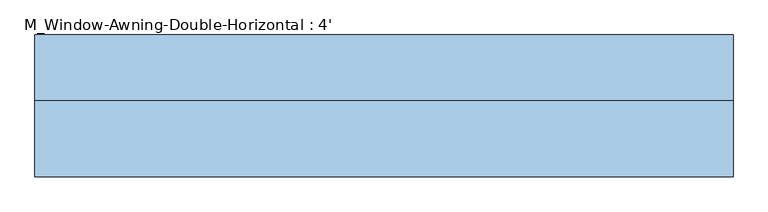
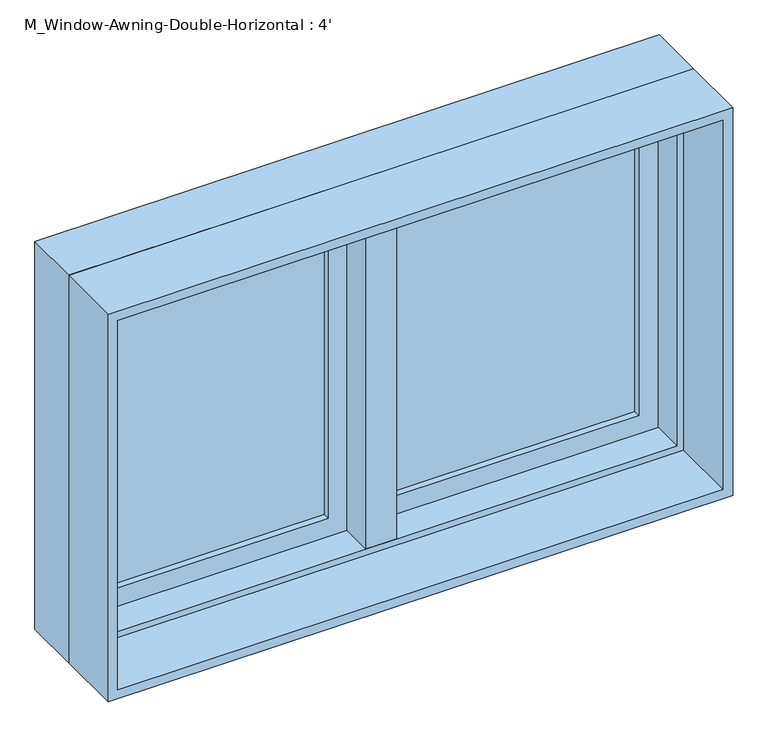
"""IFC4 building model written with IfcOpenShell, lengths in millimetres: window geometry, M_Window-Awning-Double-Horizontal : 4'."""

from ifc_helpers import new_model, si_unit, frame, origin, place, context, project, spatial, polyline, outline, extrude, faceted_brep, source, transform, mapped, element, save


def m_window_awning_double_horizontal_4_8afcb0b2(model_context):
    return source(origin(), model_context, "Body", "SolidModel", [
        faceted_brep([(577.85, 82.55, 1668.25), (577.85, 19.05, 1668.25), (-577.85, 19.05, 1668.25), (-577.85, 82.55, 1668.25), (596.9, 133.35, 1687.3), (596.9, 82.55, 1687.3), (-596.9, 82.55, 1687.3), (-596.9, 133.35, 1687.3), (609.6, 19.05, 1700.0), (609.6, 133.35, 1700.0), (-609.6, 133.35, 1700.0), (-609.6, 19.05, 1700.0), (-577.85, 19.05, 931.75), (-577.85, 82.55, 931.75), (-596.9, 82.55, 912.7), (-596.9, 133.35, 912.7), (-609.6, 133.35, 900.0), (-609.6, 19.05, 900.0), (577.85, 19.05, 931.75), (577.85, 82.55, 931.75), (596.9, 82.55, 912.7), (596.9, 133.35, 912.7), (609.6, 133.35, 900.0), (609.6, 19.05, 900.0)], [[[0, 1, 2, 3]], [[4, 5, 6, 7]], [[8, 9, 10, 11]], [[3, 2, 12, 13]], [[7, 6, 14, 15]], [[11, 10, 16, 17]], [[13, 12, 18, 19]], [[15, 14, 20, 21]], [[17, 16, 22, 23]], [[11, 17, 23, 8], [1, 18, 12, 2]], [[19, 18, 1, 0]], [[5, 20, 14, 6], [3, 13, 19, 0]], [[21, 20, 5, 4]], [[23, 22, 9, 8]], [[9, 22, 16, 10], [7, 15, 21, 4]]]),
        extrude(outline(polyline([(1700.0, -609.6), (900.0, -609.6), (900.0, 609.6), (1700.0, 609.6), (1700.0, -609.6)]), holes=[polyline([(1680.95, 590.55), (919.05, 590.55), (919.05, -590.55), (1680.95, -590.55), (1680.95, 590.55)])]), frame((0.0, -114.3, 0.0), z_axis=(0.0, 1.0, 0.0), x_axis=(0.0, 0.0, 1.0)), (0.0, 0.0, 1.0), 133.35),
        extrude(outline(polyline([(912.7, 596.9), (1687.3, 596.9), (1687.3, 9.525), (912.7, 9.525), (912.7, 596.9)]), holes=[polyline([(969.85, 66.675), (1630.15, 66.675), (1630.15, 539.75), (969.85, 539.75), (969.85, 66.675)])]), frame((0.0, 82.55, 0.0), z_axis=(0.0, 1.0, 0.0), x_axis=(0.0, 0.0, 1.0)), (0.0, 0.0, 1.0), 44.45),
        extrude(outline(polyline([(1687.3, -596.9), (912.7, -596.9), (912.7, -9.525), (1687.3, -9.525), (1687.3, -596.9)]), holes=[polyline([(1630.15, -66.675), (969.85, -66.675), (969.85, -539.75), (1630.15, -539.75), (1630.15, -66.675)])]), frame((0.0, 82.55, 0.0), z_axis=(0.0, 1.0, 0.0), x_axis=(0.0, 0.0, 1.0)), (0.0, 0.0, 1.0), 44.45),
        extrude(outline(polyline([(539.75, 114.3), (539.75, 107.95), (66.675, 107.95), (66.675, 114.3), (539.75, 114.3)])), frame((0.0, 0.0, 969.85), z_axis=(0.0, 0.0, 1.0), x_axis=(1.0, 0.0, 0.0)), (0.0, 0.0, 1.0), 660.3),
        extrude(outline(polyline([(66.675, 95.25), (66.675, 101.6), (539.75, 101.6), (539.75, 95.25), (66.675, 95.25)])), frame((0.0, 0.0, 969.85), z_axis=(0.0, 0.0, 1.0), x_axis=(1.0, 0.0, 0.0)), (0.0, 0.0, 1.0), 660.3),
        extrude(outline(polyline([(-66.675, 114.3), (-66.675, 107.95), (-539.75, 107.95), (-539.75, 114.3), (-66.675, 114.3)])), frame((0.0, 0.0, 969.85), z_axis=(0.0, 0.0, 1.0), x_axis=(1.0, 0.0, 0.0)), (0.0, 0.0, 1.0), 660.3),
        extrude(outline(polyline([(-539.75, 95.25), (-539.75, 101.6), (-66.675, 101.6), (-66.675, 95.25), (-539.75, 95.25)])), frame((0.0, 0.0, 969.85), z_axis=(0.0, 0.0, 1.0), x_axis=(1.0, 0.0, 0.0)), (0.0, 0.0, 1.0), 660.3),
        faceted_brep([(9.525, 133.35, 1687.3), (-9.525, 133.35, 1687.3), (-9.525, 82.55, 1687.3), (9.525, 82.55, 1687.3), (9.525, 133.35, 912.7), (9.525, 82.55, 912.7), (-9.525, 82.55, 912.7), (-9.525, 133.35, 912.7), (-9.525, 82.55, 931.75), (-9.525, 82.55, 1668.25), (-30.1625, 82.55, 931.75), (-30.1625, 82.55, 1668.25), (-30.1625, 19.05, 931.75), (-30.1625, 19.05, 1668.25), (30.1625, 19.05, 931.75), (30.1625, 19.05, 1668.25), (30.1625, 82.55, 931.75), (30.1625, 82.55, 1668.25), (9.525, 82.55, 931.75), (9.525, 82.55, 1668.25)], [[[0, 1, 2, 3]], [[4, 5, 6, 7]], [[1, 0, 4, 7]], [[2, 1, 7, 6, 8, 9]], [[9, 8, 10, 11]], [[11, 10, 12, 13]], [[13, 12, 14, 15]], [[15, 14, 16, 17]], [[17, 16, 18, 19]], [[0, 3, 19, 18, 5, 4]], [[18, 8, 6, 5]], [[9, 19, 3, 2]], [[8, 18, 16, 14, 12, 10]], [[19, 9, 11, 13, 15, 17]]]),
    ])


if __name__ == "__main__":
    model = new_model("IFC4")
    model_context = context("Model", 3, world=origin())
    ifc_project = project(units=[si_unit("LENGTHUNIT", "METRE", prefix="MILLI")], contexts=[model_context])
    site = spatial("IfcSite", under=ifc_project)
    building = spatial("IfcBuilding", under=site)
    placement = place(None, origin())
    m_window_awning_double_horizontal_4_shape = m_window_awning_double_horizontal_4_8afcb0b2(model_context)
    element("IfcWindow", 1, ObjectType="M_Window-Awning-Double-Horizontal : 4'", at=placement, inside=building, context=model_context, shape_type="MappedRepresentation", body=[
        mapped(m_window_awning_double_horizontal_4_shape, transform((0.0, 0.0, 0.0), x_axis=(1.0, 0.0, 0.0), y_axis=(0.0, 1.0, 0.0), z_axis=(0.0, 0.0, 1.0))),
    ])
    save(model, "model.ifc")

# Revit data of these elements
# Type "M_Window-Awning-Double-Horizontal : 4'"
#   Type Mark = "28"
#   Fire Rating = "0.5h"
#   Assembly Code = "B2020100"
#   Analytic Construction = "Double glazing - domestic"
#   Window Inset [instance default] = 0' - 0"
#   Wall Thickness [instance default] = 0' - 5.90551"
#   Interior Wall Closure [instance default] = 0' - 2.15551"
#   Half Width = 2' - 0"
#   Visual Light Transmittance = 0.81
#   Thermal Resistance (R) = 0.319569 (m²·K)/W
#   Solar Heat Gain Coefficient = 0.76
#   Rough Width = 4' - 0.59055"
#   Rough Height = 2' - 8.08661"
#   Height = 2' - 7.49606"
#   Heat Transfer Coefficient (U) = 3.12929 W/(m²·K)
#   Frame Extension [instance default] = 0' - 0 1/4"
#   Exterior Wall Closure [instance default] = 0' - 1 1/4"
#   Extension Jamb [instance default] = 0' - 2.15551"
#   Default Sill Height = 2' - 11.43307"
#   Width = 4' - 0"
#   Muntin Visibility = yes
#   Interior Trim Visibility [instance default] = yes
#   Exterior Trim Visibility [instance default] = yes
#   Extension Jamb Visibility [instance default] = yes
#   Interior Trim Material = Wood - Stained
#   Muntin Pattern = M_Muntin Pattern_2x2 : M_Muntin Pattern_2x2
#   Interior Trim = M_Trim-Window-Interior-Flat : Picture Frame
#   Interior Frame Material = Wood - Stained
#   Glass Panel Material = Glass
#   Exterior Trim Material = Clad - White
#   Exterior Trim = M_Trim-Window-Exterior-Flat : with Sill
#   Exterior Frame Material = Clad - White
#   Wall Closure = (empty or 0)
# Element 1 (IfcWindow, "M_Window-Awning-Double-Horizontal : 4'")
#   Wall Thickness = 0' - 9"
#   Extension Jamb = 0' - 5 1/4"
#   Materials on its faces: "Wood - Stained", "Glass", "Clad - White"
# Materials
#   "Wood - Stained": class "Wood", colour RGB 224 178 126, transparency 0, Cost = 0
#   "Glass": class "Glass", colour RGB 0 128 192, transparency 0.9, Description = "Soda Lime Glass", Cost = 0
#   "Clad - White": class "Wood", colour RGB 242 242 238, transparency 0, Cost = 0
